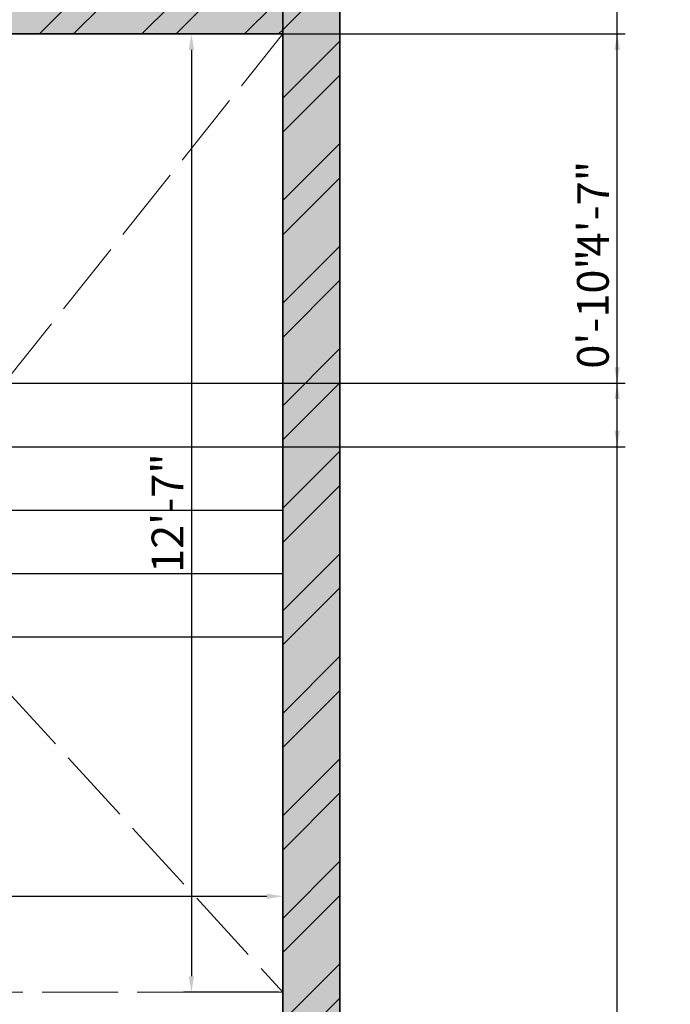
# Model space of a CAD drawing. Units: inches. Extents: x 1804 to 3296, y 909 to 2477.
# Tile 9 of 31: x 2275 to 2378, y 1174 to 1329. Entities that reach past the tile are written whole.
import ezdxf

# ---------------------------------------------------------------- set-up
doc = ezdxf.new("R2010")
doc.units = ezdxf.units.IN
doc.linetypes.add('ACAD_ISO02W100', pattern=[15, 12, -3])
for name, color, linetype, lineweight in [('A-ANNO-DIMS', 2, 'Continuous', 18), ('A-ANNO-TTLB', 156, 'Continuous', 35), ('A-FLOR-STRS', 7, 'Continuous', 25), ('A-FLOR-STRS-OVHD', 8, 'ACAD_ISO02W100', 18), ('A-GLAZ-OVHD', 130, 'ACAD_ISO02W100', 18), ('A-WALL-PATT', 10, 'Continuous', 13), ('C-PROP', 7, 'Continuous', 25), ('WALL', 10, 'Continuous', 35)]:
    doc.layers.add(name, color=color, linetype=linetype, lineweight=lineweight)
doc.styles.get("Standard").update_dxf_attribs({"font": 'arial.ttf'})
doc.dimstyles.new('ISO-25', dxfattribs={"dimtxt": 5, "dimasz": 2.5, "dimexe": 1.25, "dimexo": 0.625, "dimtad": 1, "dimdec": 0, "dimlunit": 4, "dimtxsty": 'Standard', "dimcen": 2.5, "dimadec": 0, "dimazin": 0, "dimtfac": 1, "dimtdec": 0, "dimtmove": 0, "dimatfit": 3, "dimfxl": 1, "dimarcsym": 0})
pattern_1 = [(45, (0, 196.207), (-8.08223, 8.08223), []), (45, (5.388, 196.207), (-8.08223, 8.08223), [])]

# ---------------------------------------------------------------- blocks, each defined once
blk = doc.blocks.new('*D18')
at = {"layer": 'A-ANNO-DIMS', "color": 0, "lineweight": -2, "transparency": 16777216}
for p, q in [((2315.91, 1326.69), (2300.88, 1326.69)), ((2302.13, 1324.19), (2302.13, 1178.13)), ((2315.91, 1175.63), (2300.88, 1175.63))]:
    blk.add_line(p, q, dxfattribs=at)
at = {"layer": 'A-ANNO-DIMS', "color": 0, "lineweight": 100, "transparency": 16777216}
for points in [[(2301.72, 1324.19), (2302.55, 1324.19), (2302.13, 1326.69)], [(2301.72, 1178.13), (2302.55, 1178.13), (2302.13, 1175.63)]]:
    blk.add_solid(points, dxfattribs=at)
at = {"layer": 'Defpoints', "color": 0, "lineweight": 100, "transparency": 16777216}
for p in [(2316.54, 1326.69), (2302.13, 1175.63), (2316.54, 1175.63)]:
    blk.add_point(p, dxfattribs=at)
at = {"layer": 'A-ANNO-DIMS', "color": 0, "transparency": 16777216, "insert": (2299, 1251.16), "char_height": 5, "attachment_point": 5, "rotation": 90}
blk.add_mtext('12\'-7"', dxfattribs=at)
blk = doc.blocks.new('*D19')
at = {"layer": 'A-ANNO-DIMS', "color": 0, "lineweight": -2, "transparency": 16777216}
for p, q in [((2158.58, 1176.26), (2158.58, 1192)), ((2161.08, 1190.75), (2314.04, 1190.75)), ((2316.54, 1176.26), (2316.54, 1192))]:
    blk.add_line(p, q, dxfattribs=at)
at = {"layer": 'A-ANNO-DIMS', "color": 0, "lineweight": 100, "transparency": 16777216}
for points in [[(2161.08, 1191.16), (2161.08, 1190.33), (2158.58, 1190.75)], [(2314.04, 1191.16), (2314.04, 1190.33), (2316.54, 1190.75)]]:
    blk.add_solid(points, dxfattribs=at)
at = {"layer": 'Defpoints', "color": 0, "lineweight": 100, "transparency": 16777216}
for p in [(2316.54, 1190.75), (2158.58, 1175.63), (2316.54, 1175.63)]:
    blk.add_point(p, dxfattribs=at)
at = {"layer": 'A-ANNO-DIMS', "color": 0, "transparency": 16777216, "insert": (2237.56, 1193.93), "char_height": 5, "attachment_point": 5}
blk.add_mtext('13\'-2"', dxfattribs=at)
blk = doc.blocks.new('*D53')
at = {"layer": 'A-ANNO-DIMS', "color": 0, "lineweight": -2, "transparency": 16777216}
for p, q in [((2326.16, 1793.38), (2370.49, 1793.38)), ((2369.24, 1140.57), (2369.24, 1790.88)), ((2326.16, 1138.07), (2370.49, 1138.07))]:
    blk.add_line(p, q, dxfattribs=at)
at = {"layer": 'A-ANNO-DIMS', "color": 0, "lineweight": 100, "transparency": 16777216}
for points in [[(2368.82, 1790.88), (2369.65, 1790.88), (2369.24, 1793.38)], [(2368.82, 1140.57), (2369.65, 1140.57), (2369.24, 1138.07)]]:
    blk.add_solid(points, dxfattribs=at)
at = {"layer": 'Defpoints', "color": 0, "lineweight": 100, "transparency": 16777216}
for p in [(2325.54, 1793.38), (2369.24, 1793.38), (2325.54, 1138.07)]:
    blk.add_point(p, dxfattribs=at)
at = {"layer": 'A-ANNO-DIMS', "color": 0, "transparency": 16777216, "insert": (2366.03, 1465.72), "char_height": 5, "attachment_point": 5, "rotation": 90}
blk.add_mtext('54\'-7 1/2"', dxfattribs=at)
blk = doc.blocks.new('*D72')
at = {"layer": 'A-ANNO-DIMS', "color": 0, "lineweight": -2, "transparency": 16777216}
for p, q in [((2369.24, 1271.63), (2369.24, 1292.56)), ((2159.2, 1271.63), (2370.49, 1271.63)), ((2369.24, 1264.13), (2369.24, 1269.13)), ((2159.2, 1261.63), (2370.49, 1261.63))]:
    blk.add_line(p, q, dxfattribs=at)
at = {"layer": 'A-ANNO-DIMS', "color": 0, "lineweight": 100, "transparency": 16777216}
for points in [[(2368.82, 1269.13), (2369.65, 1269.13), (2369.24, 1271.63)], [(2368.82, 1264.13), (2369.65, 1264.13), (2369.24, 1261.63)]]:
    blk.add_solid(points, dxfattribs=at)
at = {"layer": 'Defpoints', "color": 0, "lineweight": 100, "transparency": 16777216}
for p in [(2158.58, 1271.63), (2369.24, 1271.63), (2158.58, 1261.63)]:
    blk.add_point(p, dxfattribs=at)
at = {"layer": 'A-ANNO-DIMS', "color": 0, "transparency": 16777216, "insert": (2366.06, 1283.35), "char_height": 5, "attachment_point": 5, "rotation": 90}
blk.add_mtext('0\'-10"', dxfattribs=at)
blk = doc.blocks.new('*D73')
at = {"layer": 'A-ANNO-DIMS', "color": 0, "lineweight": -2, "transparency": 16777216}
for p, q in [((2272.59, 1272.26), (2272.59, 1874.99)), ((2275.09, 1873.74), (2314.04, 1873.74)), ((2316.54, 1272.26), (2316.54, 1874.99))]:
    blk.add_line(p, q, dxfattribs=at)
at = {"layer": 'A-ANNO-DIMS', "color": 0, "lineweight": 100, "transparency": 16777216}
for points in [[(2275.09, 1874.15), (2275.09, 1873.32), (2272.59, 1873.74)], [(2314.04, 1874.15), (2314.04, 1873.32), (2316.54, 1873.74)]]:
    blk.add_solid(points, dxfattribs=at)
at = {"layer": 'Defpoints', "color": 0, "lineweight": 100, "transparency": 16777216}
for p in [(2316.54, 1873.74), (2272.59, 1271.63), (2316.54, 1271.63)]:
    blk.add_point(p, dxfattribs=at)
at = {"layer": 'A-ANNO-DIMS', "color": 0, "transparency": 16777216, "insert": (2294.56, 1876.92), "char_height": 5, "attachment_point": 5}
blk.add_mtext('3\'-8"', dxfattribs=at)
blk = doc.blocks.new('*D74')
at = {"layer": 'A-ANNO-DIMS', "color": 0, "lineweight": -2, "transparency": 16777216}
for p, q in [((2273.21, 1326.69), (2370.49, 1326.69)), ((2369.24, 1274.13), (2369.24, 1324.19)), ((2273.21, 1271.63), (2370.49, 1271.63))]:
    blk.add_line(p, q, dxfattribs=at)
at = {"layer": 'A-ANNO-DIMS', "color": 0, "lineweight": 100, "transparency": 16777216}
for points in [[(2368.82, 1324.19), (2369.65, 1324.19), (2369.24, 1326.69)], [(2368.82, 1274.13), (2369.65, 1274.13), (2369.24, 1271.63)]]:
    blk.add_solid(points, dxfattribs=at)
at = {"layer": 'Defpoints', "color": 0, "lineweight": 100, "transparency": 16777216}
for p in [(2272.59, 1326.69), (2369.24, 1326.69), (2272.59, 1271.63)]:
    blk.add_point(p, dxfattribs=at)
at = {"layer": 'A-ANNO-DIMS', "color": 0, "transparency": 16777216, "insert": (2366.11, 1299.16), "char_height": 5, "attachment_point": 5, "rotation": 90}
blk.add_mtext('4\'-7"', dxfattribs=at)

msp = doc.modelspace()

# ---------------------------------------------------------------- hatches: boundary and pattern name
at = {"layer": 'A-ANNO-TTLB'}
h = msp.add_hatch(color=256, dxfattribs=at)
h.dxf.hatch_style = 1
h.paths.add_polyline_path([(3294.53, 2476.54), (1803.79, 2476.54), (1805.43, 909.47), (3296.17, 909.47)])
h.paths.add_polyline_path([(1811, 914.33), (1812.79, 2467.54), (3285.53, 2467.54), (3283.74, 914.33)], flags=16)
h.paths.add_polyline_path([(1925.58, 1062.77), (1925.58, 1138.07), (1925.58, 1539.88), (1925.58, 1793.38), (1925.58, 1830.04), (2325.54, 1830.04), (2325.54, 1793.38), (2325.54, 1586.42), (2325.54, 1138.07), (2325.54, 1062.77)], flags=0)
h.paths.add_polyline_path([(1997.22, 1029.4), (2008.85, 1037.96), (2008.85, 1020.84)], flags=0)
h.paths.add_polyline_path([(1934.58, 1138.07), (1934.58, 1147.07), (2078.77, 1147.07), (2078.77, 1138.07), (2060.94, 1138.07)], flags=0)
h.paths.add_polyline_path([(1944.35, 1138.07), (1944.35, 1147.07), (2056.05, 1147.07), (2056.05, 1138.07)], flags=0)
h.paths.add_polyline_path([(2222.24, 1037.96), (2233.87, 1029.4), (2222.24, 1020.84)], flags=0)
h.paths.add_polyline_path([(2061.94, 1139.07), (2061.94, 1146.07), (2077.77, 1146.07), (2077.77, 1139.07)], flags=0)
h.paths.add_polyline_path([(2149.58, 1138.07), (2149.58, 1269.44), (2158.58, 1269.44), (2158.58, 1326.69), (2149.58, 1326.69), (2149.58, 1340.94), (2139.6, 1340.94), (2139.6, 1434.25), (2149.58, 1434.25), (2149.58, 1447.36), (2158.58, 1447.36), (2158.58, 1423.87), (2158.58, 1408.06), (2198.46, 1408.06), (2198.46, 1412.56), (2282.65, 1412.56), (2282.65, 1465.94), (2316.54, 1465.94), (2316.54, 1590.92), (2192.86, 1590.92), (2192.86, 1595.3), (2291.17, 1595.3), (2291.17, 1590.92), (2316.54, 1590.92), (2316.54, 1784.38), (2300.24, 1784.38), (2300.24, 1757.47), (2268, 1757.47), (2268, 1681.04), (2180.87, 1681.04), (2180.87, 1757.47), (2148.63, 1757.47), (2148.63, 1784.38), (2119.08, 1784.38), (2119.08, 1585.58), (2114.58, 1585.58), (2114.58, 1784.38), (2064.11, 1784.38), (2046.28, 1784.38), (2046.28, 1760.38), (1958.58, 1760.38), (1958.58, 1664.38), (1934.58, 1664.38), (1934.58, 1784.38), (1934.58, 1793.38), (2046.28, 1793.38), (2064.11, 1793.38), (2119.08, 1793.38), (2230.78, 1793.38), (2230.78, 1784.38), (2268, 1784.38), (2300.24, 1784.38), (2316.54, 1784.38), (2316.54, 1590.92), (2316.54, 1373.73), (2316.54, 1138.07)], flags=0)
h.paths.add_polyline_path([(2209.19, 1166.63), (2209.19, 1175.63), (2158.58, 1175.63), (2209.19, 1223.63), (2209.19, 1231.63), (2183.88, 1231.63), (2183.88, 1301.66), (2242.59, 1301.66), (2242.59, 1326.69), (2316.54, 1326.69), (2272.59, 1271.63), (2272.59, 1223.63), (2316.54, 1175.63), (2272.59, 1175.63), (2272.59, 1166.63)], flags=0)
h.paths.add_polyline_path([(1947.77, 1345.22), (1947.77, 1457.48), (1991.2, 1457.48), (1991.2, 1451.7), (1991.2, 1352.18), (1991.2, 1345.22)], flags=0)
h.paths.add_polyline_path([(2209.19, 1271.63), (2262.59, 1271.63), (2262.59, 1311.85), (2272.59, 1301.66), (2272.59, 1271.63), (2269.92, 1269.63), (2270.59, 1269.63), (2270.59, 1225.63), (2211.19, 1225.63), (2211.19, 1269.63), (2211.86, 1269.63)], flags=0)
h.paths.add_polyline_path([(2000.34, 1378.21), (2000.34, 1429.71), (2025.22, 1429.71), (2025.22, 1378.21)], flags=0)
h.paths.add_polyline_path([(2001.34, 1379.21), (2001.34, 1428.71), (2024.22, 1428.71), (2024.22, 1379.21)], flags=0)
h.paths.add_polyline_path([(2012.34, 1390.21), (2012.34, 1417.71), (2013.22, 1417.71), (2013.22, 1390.21)], flags=0)
h.paths.add_polyline_path([(2237.56, 1331.19), (2237.56, 1340.18), (2238.62, 1340.18), (2238.62, 1386.84), (2241.04, 1386.84), (2242.06, 1386.84), (2242.06, 1408.06), (2316.54, 1331.19)], flags=0)
h.paths.add_polyline_path([(1953.73, 1464.35), (1953.73, 1498.59), (1981.74, 1498.59), (1981.74, 1464.35)], flags=0)
h.paths.add_polyline_path([(1987.63, 1462.08), (1987.63, 1500.95), (2104.07, 1500.95), (2104.07, 1462.08), (2099.27, 1462.08), (1993.6, 1462.08)], flags=0)
h.paths.add_polyline_path([(1956.06, 1481.47, -1), (1979.41, 1481.47, -1)], flags=0)
edge = h.paths.add_edge_path(flags=0)
edge.add_ellipse((2299.53, 1438.37), major_axis=(0.31, 21.36), ratio=0.670333, start_angle=0, end_angle=360)
h.paths.add_polyline_path([(2297.39, 1438.37, -1), (2301.67, 1438.37, -1)], flags=0)
h.paths.add_polyline_path([(2591.54, 1163.23), (2591.54, 1179.38), (2591.54, 1379.68), (2591.54, 1395.84), (2734.5, 1395.84), (2734.5, 1379.68), (2734.5, 1179.38), (2734.5, 1163.23)], flags=0)
h.paths.add_polyline_path([(2592.54, 1164.23), (2592.54, 1166.23), (2733.5, 1166.23), (2733.5, 1164.23)], flags=0)
h.paths.add_polyline_path([(2592.54, 1180.38), (2592.54, 1378.68), (2733.5, 1378.68), (2733.5, 1180.38)], flags=0)
h.paths.add_polyline_path([(2593.54, 1181.38), (2593.54, 1377.68), (2732.5, 1377.68), (2732.5, 1181.38)], flags=0)
h.paths.add_polyline_path([(2594.54, 1182.38), (2594.54, 1376.68), (2731.5, 1376.68), (2731.5, 1182.38)], flags=0)
h.paths.add_polyline_path([(1936.95, 1697.46), (1936.95, 1736.46), (1955.41, 1736.46), (1955.41, 1697.46)], flags=0)
h.paths.add_polyline_path([(1938.48, 1718.36), (1938.48, 1734.92), (1953.65, 1734.92), (1953.65, 1718.36)], flags=0)
h.paths.add_polyline_path([(1944.75, 1726.64, -1), (1947.37, 1726.64, -1)], flags=0)
h.paths.add_polyline_path([(2592.54, 1394.84), (2733.5, 1394.84), (2733.5, 1392.84), (2592.54, 1392.84)], flags=0)
h.paths.add_polyline_path([(1976.61, 1762.5), (1976.61, 1781.44), (2012.79, 1781.44), (2012.79, 1762.5)], flags=0)
h.paths.add_polyline_path([(1979.57, 1771.97, -1), (1991.39, 1771.97, -1)], flags=0)
h.paths.add_polyline_path([(1995.36, 1771.97, -1), (2007.18, 1771.97, -1)], flags=0)
h.paths.add_polyline_path([(2251.51, 1744.53), (2268, 1730.05), (2251.51, 1730.05)], flags=0)
h.paths.add_polyline_path([(2047.28, 1785.38), (2047.28, 1792.38), (2063.11, 1792.38), (2063.11, 1785.38)], flags=0)
h.paths.add_polyline_path([(2155.08, 1770.92, -1), (2174.42, 1770.92, -1)], flags=0)
h.paths.add_polyline_path([(2188.59, 1758.27), (2188.59, 1772.81), (2222.3, 1772.81), (2222.3, 1758.27)], flags=0)
h.paths.add_polyline_path([(2223.97, 1758.27), (2223.97, 1772.81), (2257.68, 1772.81), (2257.68, 1758.27)], flags=0)
h.paths.add_polyline_path([(2274.45, 1770.92, -1), (2293.8, 1770.92, -1)], flags=0)
h.paths.add_polyline_path([(2591.54, 1582.09), (2591.54, 1782.39), (2734.5, 1782.39), (2734.5, 1582.09)], flags=0)
h.paths.add_polyline_path([(2592.54, 1583.09), (2592.54, 1781.39), (2733.5, 1781.39), (2733.5, 1583.09)], flags=0)
h.paths.add_polyline_path([(2593.54, 1584.09), (2593.54, 1780.39), (2732.5, 1780.39), (2732.5, 1584.09)], flags=0)
h.paths.add_polyline_path([(2594.54, 1585.09), (2594.54, 1779.39), (2731.5, 1779.39), (2731.5, 1585.09)], flags=0)
h.paths.add_polyline_path([(1922.17, 1978.79), (1922.17, 2295.08), (1922.17, 2296.08), (2115.67, 2296.08), (2115.67, 2384.31), (2115.67, 2385.31), (2322.12, 2385.31), (2323.12, 2385.31), (2323.12, 1979.79), (2323.12, 1978.79), (1923.17, 1978.79)], flags=0)
h.paths.add_polyline_path([(1922.17, 1978.79), (1922.17, 2051.31), (1922.17, 2214.86), (1922.17, 2296.08), (2115.67, 2296.08), (2115.67, 2385.31), (2323.12, 2385.31), (2323.12, 2280.42), (2323.12, 1978.79), (2115.67, 1978.79)], flags=0)
h.paths.add_polyline_path([(1923.17, 1979.79), (1923.17, 2050.31), (2115.67, 2050.31), (2115.67, 2051.31), (1923.17, 2051.31), (1923.17, 2213.86), (1923.17, 2214.86), (1923.17, 2295.08), (1990.02, 2295.08), (1990.02, 2214.86), (1991.02, 2214.86), (1991.02, 2295.08), (2115.67, 2295.08), (2115.67, 1979.79), (2116.67, 1979.79), (2116.67, 2304.18), (2116.67, 2384.31), (2322.12, 2384.31), (2322.12, 2280.42), (2322.12, 1979.79), (2115.67, 1979.79)], flags=0)
h.paths.add_polyline_path([(2972.46, 1192.5), (2972.46, 1196.92), (2995.47, 1196.92), (2995.47, 1255.47), (2995.09, 1255.47), (2987.42, 1249.39), (2980.08, 1255.47), (2978.05, 1255.47), (2978.05, 1257.24), (2995.47, 1257.24), (2995.47, 1261.58), (3015.37, 1261.58), (3015.37, 1333.28), (3015.37, 1414.4), (3032.82, 1414.4), (3032.82, 1333.28), (3032.82, 1261.58), (3052.66, 1261.58), (3052.66, 1255.47), (3079.86, 1255.47), (3078.72, 1254.57), (3081.47, 1252.29), (3078.56, 1249.99), (3075.81, 1252.26), (3072.57, 1249.69), (3070.36, 1251.52), (3067.67, 1249.39), (3060.34, 1255.47), (3052.66, 1255.47), (3052.66, 1196.92), (3054.58, 1196.92), (3074, 1196.92), (3074, 1192.5), (3052.66, 1192.5), (2995.47, 1192.5)], flags=0)
h.paths.add_polyline_path([(2490.75, 1979.27), (2490.75, 1980.27), (2596.87, 1980.27), (2596.87, 2051.8), (2596.87, 2052.8), (2596.87, 2216.35), (2596.87, 2297.57), (2717.32, 2297.57), (2710.57, 2305.62), (2724.07, 2305.62), (2717.32, 2297.57), (2782.37, 2297.57), (2782.37, 2395.8), (3006.82, 2395.8), (3006.82, 1981.27), (3093.73, 1981.27), (3093.73, 1980.27), (3047.51, 1980.27), (3046.37, 1979.37), (3049.11, 1977.1), (3046.2, 1974.79), (3043.46, 1977.07), (3040.21, 1974.49), (3038, 1976.32), (3035.32, 1974.2), (3027.98, 1980.27), (2871.83, 1980.27), (2871.83, 1981.27), (2791.37, 1981.27), (2791.37, 2050.8), (2597.87, 2050.8), (2597.87, 1980.27), (2597.87, 1979.27), (2546.27, 1979.27), (2545.12, 1978.37), (2547.87, 1976.1), (2544.96, 1973.79), (2542.22, 1976.07), (2538.97, 1973.49), (2536.76, 1975.32), (2534.07, 1973.2), (2526.74, 1979.27)], flags=0)
h.paths.add_polyline_path([(2597.87, 2051.8), (2606.87, 2051.8), (2606.87, 2258.39), (2597.87, 2258.39), (2597.87, 2296.57), (2606.87, 2296.57), (2606.87, 2262.39), (2782.37, 2262.39), (2782.37, 2296.57), (2790.37, 2296.57), (2790.37, 2262.39), (2791.37, 2262.39), (2791.37, 2305.67), (2791.37, 2385.8), (2996.82, 2385.8), (2996.82, 2339.85), (3006.82, 2339.85), (3006.82, 2250.12), (2997.82, 2250.12), (2997.82, 1981.27), (2996.82, 1981.27), (2872.83, 1981.27), (2872.83, 1991.8), (2871.83, 1991.8), (2871.83, 2050.8), (2790.37, 2050.8), (2597.87, 2050.8)], flags=0)
h.paths.add_polyline_path([(2179.93, 2153.92), (2179.93, 2353.97), (2259.98, 2353.97), (2259.98, 2153.92)], flags=0)
h.paths.add_polyline_path([(2180.93, 2154.92), (2180.93, 2352.97), (2258.98, 2352.97), (2258.98, 2154.92)], flags=0)
h.paths.add_polyline_path([(2960.87, 1608.49), (2960.87, 1753.62), (3070.9, 1753.62), (3070.9, 1608.49)], flags=0)
h.paths.add_polyline_path([(2961.87, 1609.49), (2961.87, 1752.62), (3069.9, 1752.62), (3069.9, 1609.49)], flags=0)
h.paths.add_polyline_path([(2962.87, 1610.49), (2962.87, 1751.62), (3068.9, 1751.62), (3068.9, 1610.49)], flags=0)
h.paths.add_polyline_path([(2963.87, 1611.49), (2963.87, 1750.62), (3067.9, 1750.62), (3067.9, 1611.49)], flags=0)
h.paths.add_polyline_path([(2782.37, 2051.8), (2782.37, 2216.32), (2791.37, 2216.32), (2791.37, 2051.8), (2872.83, 2051.8), (2872.83, 2068.56), (2884.67, 2068.56), (2884.67, 2085.33), (2896.51, 2085.33), (2896.51, 2102.09), (2908.36, 2102.09), (2908.36, 2118.85), (2920.2, 2118.85), (2920.2, 2135.62), (2932.05, 2135.62), (2932.05, 2145.3), (2925.08, 2145.3), (2925.08, 2203.2), (2996.82, 2203.2), (2996.82, 2145.3), (2953.82, 2145.3), (2872.83, 2051.8), (2790.37, 2051.8)], flags=0)
h.paths.add_polyline_path([(2717.32, 2238.65), (2710.57, 2246.7), (2724.07, 2246.7)], flags=0)
h.paths.add_polyline_path([(2003.09, 1122.79), (2017.16, 1122.79), (2017.16, 1138.74), (2003.09, 1138.74)], flags=8)
h.paths.add_polyline_path([(2174.76, 1792.72), (2188.83, 1792.72), (2188.83, 1808.66), (2174.76, 1808.66)], flags=8)
h.paths.add_polyline_path([(1987.95, 1792.51), (2002.02, 1792.51), (2002.02, 1808.45), (1987.95, 1808.45)], flags=8)
h.paths.add_polyline_path([(2148.79, 1289.26), (2160.46, 1289.26), (2160.46, 1305.2), (2148.79, 1305.2)], flags=8)
h.paths.add_polyline_path([(2115.36, 1133.57), (2127.04, 1133.57), (2127.04, 1149.51), (2115.36, 1149.51)], flags=8)
h.paths.add_polyline_path([(2237.58, 1421.48), (2249.25, 1421.48), (2249.25, 1437.43), (2237.58, 1437.43)], flags=8)
h.paths.add_polyline_path([(2134.99, 1584.32), (2146.66, 1584.32), (2146.66, 1600.26), (2134.99, 1600.26)], flags=8)
h.paths.add_polyline_path([(2101.95, 1557.31), (2113.62, 1557.31), (2113.62, 1573.25), (2101.95, 1573.25)], flags=8)
h.paths.add_polyline_path([(2937.85, 1156.77), (3120.41, 1156.77), (3120.41, 1185.72), (2937.85, 1185.72)], flags=8)
h.paths.add_polyline_path([(2980.71, 1786.71), (3050.06, 1786.71), (3050.06, 1802.66), (2980.71, 1802.66)], flags=8)
h.paths.add_polyline_path([(2869.28, 1661.96), (2938.62, 1661.96), (2938.62, 1690.8), (2869.28, 1690.8)], flags=8)
h.paths.add_polyline_path([(3092.27, 1674.86), (3161.62, 1674.86), (3161.62, 1690.8), (3092.27, 1690.8)], flags=8)
h.paths.add_polyline_path([(2980.71, 1674.86), (3050.06, 1674.86), (3050.06, 1690.8), (2980.71, 1690.8)], flags=8)
h.paths.add_polyline_path([(2649.07, 1678.23), (2674.53, 1678.23), (2674.53, 1714.76), (2649.07, 1714.76)], flags=8)
h.paths.add_polyline_path([(2530.84, 1981.63), (2549.13, 1981.63), (2549.13, 1997.57), (2530.84, 1997.57)], flags=8)
h.paths.add_polyline_path([(3031.29, 1981.77), (3049.58, 1981.77), (3049.58, 1997.71), (3031.29, 1997.71)], flags=8)
h.paths.add_polyline_path([(2715.38, 1911.9), (2851.54, 1911.9), (2851.54, 1940.85), (2715.38, 1940.85)], flags=8)
h.paths.add_polyline_path([(2015.23, 1927.36), (2205.42, 1927.36), (2205.42, 1956.3), (2015.23, 1956.3)], flags=8)
h.paths.add_polyline_path([(2671.84, 2057.84), (2702.75, 2057.84), (2702.75, 2073.79), (2671.84, 2073.79)], flags=8)
h.paths.add_polyline_path([(2678.5, 2316.52), (2765.26, 2316.52), (2765.26, 2332.46), (2678.5, 2332.46)], flags=8)
h.paths.add_polyline_path([(2678.48, 2271.96), (2736.41, 2271.96), (2736.41, 2287.9), (2678.48, 2287.9)], flags=8)
h.paths.add_polyline_path([(2019.2, 972.79), (2243.21, 972.79), (2243.21, 1001.74), (2019.2, 1001.74)], flags=8)
h.paths.add_polyline_path([(2097.06, 1021.56), (2132.16, 1021.56), (2132.16, 1037.51), (2097.06, 1037.51)], flags=8)
h.paths.add_polyline_path([(2182.47, 1360.48), (2207.35, 1360.48), (2207.35, 1376.42), (2182.47, 1376.42)], flags=8)
h.paths.add_polyline_path([(2261.12, 1361.77), (2295.01, 1361.77), (2295.01, 1377.71), (2261.12, 1377.71)], flags=8)
h.paths.add_polyline_path([(2245.75, 1511.51), (2278.44, 1511.51), (2278.44, 1527.46), (2245.75, 1527.46)], flags=8)
h.paths.add_polyline_path([(1991.16, 1296.29), (2060.51, 1296.29), (2060.51, 1312.23), (1991.16, 1312.23)], flags=8)
h.paths.add_polyline_path([(2187, 1651.35), (2246.71, 1651.35), (2246.71, 1667.29), (2187, 1667.29)], flags=8)
h.paths.add_polyline_path([(1976.49, 1684.81), (2068.63, 1684.81), (2068.63, 1700.76), (1976.49, 1700.76)], flags=8)
at = {"layer": 'A-WALL-PATT'}
h = msp.add_hatch(color=256, dxfattribs=at)
h.dxf.hatch_style = 1
h.paths.add_polyline_path([(2158.58, 1275.49), (2155.29, 1275.49), (2149.58, 1275.49), (2149.58, 1269.44), (2158.58, 1269.44)])
h.paths.add_polyline_path([(2158.58, 1326.69), (2149.58, 1326.69), (2149.58, 1319.33), (2155.29, 1319.33), (2158.58, 1319.33)])
h.paths.add_polyline_path([(2158.58, 1402.2), (2158.58, 1423.87), (2158.58, 1447.36), (2149.58, 1447.36), (2149.58, 1423.87), (2149.58, 1340.94), (2149.58, 1326.69), (2158.58, 1326.69), (2158.58, 1354.23)])
h.paths.add_polyline_path([(1965.87, 1658.79), (1965.87, 1679.09), (1955.57, 1679.09), (1955.57, 1658.79)], flags=9)
h.paths.add_polyline_path([(2293.18, 1677.29), (2293.18, 1697.58), (2282.88, 1697.58), (2282.88, 1677.29)], flags=9)
h.paths.add_polyline_path([(2271.13, 1545.23), (2287.53, 1545.23), (2287.53, 1555.53), (2271.13, 1555.53)], flags=9)
h.paths.add_polyline_path([(2303.26, 1488.52), (2303.26, 1508.82), (2292.95, 1508.82), (2292.95, 1488.52)], flags=9)
h.paths.add_polyline_path([(2271.13, 1393.15), (2287.53, 1393.15), (2287.53, 1403.45), (2271.13, 1403.45)], flags=9)
h.paths.add_polyline_path([(2306.48, 1361.45), (2306.48, 1377.86), (2296.18, 1377.86), (2296.18, 1361.45)], flags=9)
h.paths.add_polyline_path([(2189.9, 1340.62), (2206.31, 1340.62), (2206.31, 1350.92), (2189.9, 1350.92)], flags=9)
h.paths.add_polyline_path([(2174.54, 1361.45), (2174.54, 1377.86), (2164.23, 1377.86), (2164.23, 1361.45)], flags=9)
h.paths.add_polyline_path([(2304.24, 1240.8), (2304.24, 1261.09), (2293.94, 1261.09), (2293.94, 1240.8)], flags=9)
h.paths.add_polyline_path([(2227.19, 1188.73), (2247.49, 1188.73), (2247.49, 1199.03), (2227.19, 1199.03)], flags=9)
h.paths.add_polyline_path([(2181.93, 1144.21), (2181.93, 1160.62), (2171.63, 1160.62), (2171.63, 1144.21)], flags=9)
h.paths.add_polyline_path([(1968.21, 1333.34), (1968.21, 1353.64), (1957.91, 1353.64), (1957.91, 1333.34)], flags=9)
h.paths.add_polyline_path([(2029.78, 1203.53), (2053.95, 1203.53), (2053.95, 1213.83), (2029.78, 1213.83)], flags=9)
h.paths.add_polyline_path([(2576.51, 1671.88), (2576.51, 1692.17), (2566.21, 1692.17), (2566.21, 1671.88)], flags=9)
h.paths.add_polyline_path([(2566.99, 1269.67), (2566.99, 1289.96), (2556.68, 1289.96), (2556.68, 1269.67)], flags=9)
h.paths.add_polyline_path([(2581.85, 1269.17), (2581.85, 1289.46), (2571.54, 1289.46), (2571.54, 1269.17)], flags=9)
h.paths.add_polyline_path([(2650.71, 1409.75), (2674.89, 1409.75), (2674.89, 1420.05), (2650.71, 1420.05)], flags=9)
h.paths.add_polyline_path([(2003.09, 1122.79), (2017.16, 1122.79), (2017.16, 1138.74), (2003.09, 1138.74)], flags=9)
h.paths.add_polyline_path([(2174.76, 1792.72), (2188.83, 1792.72), (2188.83, 1808.66), (2174.76, 1808.66)], flags=9)
h.paths.add_polyline_path([(1987.95, 1792.51), (2002.02, 1792.51), (2002.02, 1808.45), (1987.95, 1808.45)], flags=9)
h.paths.add_polyline_path([(2148.79, 1289.26), (2160.46, 1289.26), (2160.46, 1305.2), (2148.79, 1305.2)], flags=9)
h.paths.add_polyline_path([(2115.36, 1133.57), (2127.04, 1133.57), (2127.04, 1149.51), (2115.36, 1149.51)], flags=9)
h.paths.add_polyline_path([(2237.58, 1421.48), (2249.25, 1421.48), (2249.25, 1437.43), (2237.58, 1437.43)], flags=9)
h.paths.add_polyline_path([(2134.99, 1584.32), (2146.66, 1584.32), (2146.66, 1600.26), (2134.99, 1600.26)], flags=9)
h.paths.add_polyline_path([(2101.95, 1557.31), (2113.62, 1557.31), (2113.62, 1573.25), (2101.95, 1573.25)], flags=9)
h.paths.add_polyline_path([(2937.85, 1156.77), (3120.41, 1156.77), (3120.41, 1185.72), (2937.85, 1185.72)], flags=9)
h.paths.add_polyline_path([(2980.71, 1786.71), (3050.06, 1786.71), (3050.06, 1802.66), (2980.71, 1802.66)], flags=9)
h.paths.add_polyline_path([(2869.28, 1661.96), (2938.62, 1661.96), (2938.62, 1690.8), (2869.28, 1690.8)], flags=9)
h.paths.add_polyline_path([(3092.27, 1674.86), (3161.62, 1674.86), (3161.62, 1690.8), (3092.27, 1690.8)], flags=9)
h.paths.add_polyline_path([(2980.71, 1674.86), (3050.06, 1674.86), (3050.06, 1690.8), (2980.71, 1690.8)], flags=9)
h.paths.add_polyline_path([(2649.07, 1678.23), (2674.53, 1678.23), (2674.53, 1714.76), (2649.07, 1714.76)], flags=9)
h.paths.add_polyline_path([(2530.84, 1981.63), (2549.13, 1981.63), (2549.13, 1997.57), (2530.84, 1997.57)], flags=9)
h.paths.add_polyline_path([(3031.29, 1981.77), (3049.58, 1981.77), (3049.58, 1997.71), (3031.29, 1997.71)], flags=9)
h.paths.add_polyline_path([(2715.38, 1911.9), (2851.54, 1911.9), (2851.54, 1940.85), (2715.38, 1940.85)], flags=9)
h.paths.add_polyline_path([(2015.23, 1927.36), (2205.42, 1927.36), (2205.42, 1956.3), (2015.23, 1956.3)], flags=9)
h.paths.add_polyline_path([(2671.84, 2057.84), (2702.75, 2057.84), (2702.75, 2073.79), (2671.84, 2073.79)], flags=9)
h.paths.add_polyline_path([(2678.5, 2316.52), (2765.26, 2316.52), (2765.26, 2332.46), (2678.5, 2332.46)], flags=9)
h.paths.add_polyline_path([(2678.48, 2271.96), (2736.41, 2271.96), (2736.41, 2287.9), (2678.48, 2287.9)], flags=9)
h.paths.add_polyline_path([(2019.2, 972.79), (2243.21, 972.79), (2243.21, 1001.74), (2019.2, 1001.74)], flags=9)
h.paths.add_polyline_path([(2097.06, 1021.56), (2132.16, 1021.56), (2132.16, 1037.51), (2097.06, 1037.51)], flags=9)
h.paths.add_polyline_path([(2182.47, 1360.48), (2207.35, 1360.48), (2207.35, 1376.42), (2182.47, 1376.42)], flags=9)
h.paths.add_polyline_path([(2261.12, 1361.77), (2295.01, 1361.77), (2295.01, 1377.71), (2261.12, 1377.71)], flags=9)
h.paths.add_polyline_path([(2245.75, 1511.51), (2278.44, 1511.51), (2278.44, 1527.46), (2245.75, 1527.46)], flags=9)
h.paths.add_polyline_path([(1991.16, 1296.29), (2060.51, 1296.29), (2060.51, 1312.23), (1991.16, 1312.23)], flags=9)
h.paths.add_polyline_path([(2187, 1651.35), (2246.71, 1651.35), (2246.71, 1667.29), (2187, 1667.29)], flags=9)
h.paths.add_polyline_path([(1976.49, 1684.81), (2068.63, 1684.81), (2068.63, 1700.76), (1976.49, 1700.76)], flags=9)
h = msp.add_hatch(dxfattribs=at)
h.set_pattern_fill('ANSI32', color=256, scale=1.2)
h.set_pattern_definition(pattern_1)
h.paths.add_polyline_path([(1934.58, 1784.38), (1934.58, 1793.38), (1925.58, 1793.38), (1925.58, 1539.88), (2119.08, 1539.88), (2119.08, 1545.58), (2114.58, 1545.58), (2114.58, 1544.38), (1934.58, 1544.38)])
h.paths.add_polyline_path([(2114.58, 1793.38), (2064.11, 1793.38), (2064.11, 1784.38), (2114.58, 1784.38)], flags=17)
h.paths.add_polyline_path([(2325.54, 1793.38), (2230.78, 1793.38), (2230.78, 1784.38), (2268, 1784.38), (2300.24, 1784.38), (2316.54, 1784.38), (2316.54, 1590.92), (2316.54, 1586.42), (2325.54, 1586.42)])
h.paths.add_polyline_path([(1944.35, 1147.07), (1934.58, 1147.07), (1934.58, 1138.07), (1944.35, 1138.07)])
h.paths.add_polyline_path([(2101.21, 1144.07, -0.01877), (2101.32, 1147.07), (2078.77, 1147.07), (2078.77, 1138.07), (2101.21, 1138.07)])
h.paths.add_polyline_path([(1934.58, 1539.88), (1925.58, 1539.88), (1925.58, 1138.07), (1934.58, 1138.07), (1934.58, 1147.07)])
h.paths.add_polyline_path([(2325.54, 1586.42), (2316.54, 1586.42), (2316.54, 1373.73), (2316.54, 1138.07), (2325.54, 1138.07), (2325.54, 1228.97)])
h.paths.add_polyline_path([(2158.58, 1423.87), (2158.58, 1447.36), (2149.58, 1447.36), (2149.58, 1423.87), (2149.58, 1340.94), (2149.58, 1326.69), (2158.58, 1326.69), (2158.58, 1354.23), (2158.58, 1402.2)])
h.paths.add_polyline_path([(2316.54, 1412.56), (2282.65, 1412.56), (2273.09, 1412.56), (2273.09, 1408.06), (2316.54, 1408.06)])
h.paths.add_polyline_path([(2273.09, 1412.56), (2242.06, 1412.56), (2242.06, 1408.06), (2273.09, 1408.06)])
h.paths.add_polyline_path([(2237.56, 1412.56), (2198.46, 1412.56), (2198.46, 1408.06), (2237.56, 1408.06)])
h.paths.add_polyline_path([(2242.06, 1408.06), (2237.56, 1408.06), (2237.56, 1386.84), (2242.06, 1386.84)])
h.paths.add_polyline_path([(2242.06, 1412.56), (2237.56, 1412.56), (2237.56, 1408.06), (2242.06, 1408.06)])
h.paths.add_polyline_path([(2158.58, 1269.44), (2149.58, 1269.44), (2149.58, 1138.07), (2158.58, 1138.07)])
h.paths.add_polyline_path([(2149.58, 1147.07), (2141.21, 1147.07), (2141.21, 1144.07), (2141.21, 1138.07), (2149.58, 1138.07)])
h.paths.add_polyline_path([(2272.59, 1175.63), (2209.19, 1175.63), (2209.19, 1166.63), (2272.59, 1166.63)])
h.paths.add_polyline_path([(2237.56, 1446.21), (2242.06, 1446.21), (2242.06, 1586.42), (2237.56, 1586.42)])
h.paths.add_polyline_path([(2242.06, 1414.58), (2237.56, 1414.58), (2237.56, 1412.56), (2242.06, 1412.56)])
h = msp.add_hatch(color=256, dxfattribs=at)
h.dxf.hatch_style = 1
h.paths.add_polyline_path([(2114.58, 1793.38), (2064.11, 1793.38), (2064.11, 1784.38), (2114.58, 1784.38)])
h.paths.add_polyline_path([(2119.08, 1793.38), (2114.58, 1793.38), (2114.58, 1585.58), (2119.08, 1585.58)])
h.paths.add_polyline_path([(2325.54, 1793.38), (2230.78, 1793.38), (2230.78, 1784.38), (2268, 1784.38), (2316.54, 1784.38), (2316.54, 1590.92), (2316.54, 1586.42), (2325.54, 1586.42)])
h.paths.add_polyline_path([(2316.54, 1331.19), (2158.58, 1331.19), (2158.58, 1326.69), (2316.54, 1326.69)])
h.paths.add_polyline_path([(2242.06, 1408.06), (2237.56, 1408.06), (2237.56, 1386.84), (2242.06, 1386.84)])
h.paths.add_polyline_path([(2242.06, 1412.56), (2237.56, 1412.56), (2237.56, 1408.06), (2242.06, 1408.06)])
h.paths.add_polyline_path([(2237.56, 1412.56), (2198.46, 1412.56), (2198.46, 1408.06), (2237.56, 1408.06)])
h.paths.add_polyline_path([(2273.09, 1412.56), (2242.06, 1412.56), (2242.06, 1408.06), (2273.09, 1408.06)])
h.paths.add_polyline_path([(2316.54, 1412.56), (2282.65, 1412.56), (2273.09, 1412.56), (2273.09, 1408.06), (2316.54, 1408.06)])
h.paths.add_polyline_path([(2325.54, 1586.42), (2316.54, 1586.42), (2316.54, 1373.73), (2316.54, 1138.07), (2325.54, 1138.07), (2325.54, 1228.97)])
h.paths.add_polyline_path([(2272.59, 1175.63), (2209.19, 1175.63), (2209.19, 1166.63), (2272.59, 1166.63)])
h = msp.add_hatch(dxfattribs=at)
h.set_pattern_fill('ANSI32', color=256, scale=1.2)
h.set_pattern_definition(pattern_1)
h.paths.add_polyline_path([(2316.54, 1331.19), (2158.58, 1331.19), (2158.58, 1326.69), (2316.54, 1326.69)])
h.paths.add_polyline_path([(2242.06, 1340.18), (2237.56, 1340.18), (2237.56, 1331.19), (2242.06, 1331.19)])
h.paths.add_polyline_path([(2242.06, 1408.06), (2237.56, 1408.06), (2237.56, 1386.84), (2242.06, 1386.84)])

# ---------------------------------------------------------------- linework, layer by layer
at = {"layer": 'A-FLOR-STRS'}
for p, q in [((2272.59, 1271.63), (2316.54, 1271.63)), ((2272.59, 1261.63), (2316.54, 1261.63)), ((2272.59, 1251.63), (2316.54, 1251.63)), ((2272.59, 1241.63), (2316.54, 1241.63)), ((2272.59, 1231.63), (2316.54, 1231.63))]:
    msp.add_line(p, q, dxfattribs=at)
at = {"layer": 'A-FLOR-STRS-OVHD'}
for p, q in [((2272.59, 1271.63), (2316.54, 1326.69)), ((2272.59, 1223.63), (2316.54, 1175.63))]:
    msp.add_line(p, q, dxfattribs=at)
at = {"layer": 'A-GLAZ-OVHD'}
msp.add_line((2158.58, 1175.63), (2316.54, 1175.63), dxfattribs=at)
at = {"layer": 'C-PROP'}
msp.add_line((2325.54, 1062.77), (2325.54, 1228.97), dxfattribs=at)
at = {"layer": 'WALL'}
for p, q in [((2325.54, 1586.42), (2325.54, 1138.07)), ((2316.54, 1373.73), (2316.54, 1138.07)), ((2158.58, 1326.69), (2316.54, 1326.69))]:
    msp.add_line(p, q, dxfattribs=at)

# ---------------------------------------------------------------- dimensions: what is measured, and where the dimension line sits
at = {"layer": 'A-ANNO-DIMS'}
for base, p1, p2, override, picture, middle in [((2316.5375, 1873.7362), (2272.5886, 1271.6342), (2316.5375, 1271.6342), {"dimdec": 1, "dimlfac": 1, "dimrnd": 0, "dimzin": 1, "dimdsep": 46, "dimlunit": 4, "dimfrac": 2}, '*D73', (2294.563, 1876.9158)), ((2316.54, 1190.75), (2158.58, 1175.63), (2316.54, 1175.63), {"dimclrd": 0, "dimclre": 0, "dimclrt": 0}, '*D19', (2237.56, 1193.93))]:
    dim = msp.add_linear_dim(base=base, p1=p1, p2=p2, dimstyle='ISO-25', override=override, dxfattribs=at)
    dim.commit()
    dim.dimension.update_dxf_attribs({"geometry": picture, "text_midpoint": middle})
for base, p1, p2, override, picture, middle in [((2369.24, 1793.38), (2325.54, 1138.07), (2325.54, 1793.38), {"dimdec": 1, "dimlfac": 1, "dimrnd": 0, "dimzin": 1, "dimdsep": 46, "dimlunit": 4, "dimfrac": 2}, '*D53', (2366.03, 1465.72)), ((2369.24, 1326.69), (2272.59, 1271.63), (2272.59, 1326.69), {"dimdec": 1, "dimlfac": 1, "dimrnd": 0, "dimzin": 1, "dimdsep": 46, "dimlunit": 4, "dimfrac": 2}, '*D74', (2366.11, 1299.16)), ((2302.13, 1175.63), (2316.54, 1326.69), (2316.54, 1175.63), {"dimclrd": 0, "dimclre": 0, "dimclrt": 0}, '*D18', (2299, 1251.16)), ((2369.24, 1271.63), (2158.58, 1261.63), (2158.58, 1271.63), {"dimdec": 1, "dimlfac": 1, "dimrnd": 0, "dimzin": 1, "dimdsep": 46, "dimlunit": 4, "dimfrac": 2}, '*D72', (2366.06, 1283.35))]:
    dim = msp.add_linear_dim(base=base, p1=p1, p2=p2, angle=90, dimstyle='ISO-25', override=override, dxfattribs=at)
    dim.commit()
    dim.dimension.update_dxf_attribs({"geometry": picture, "text_midpoint": middle})

doc.saveas('drawing.dxf')
